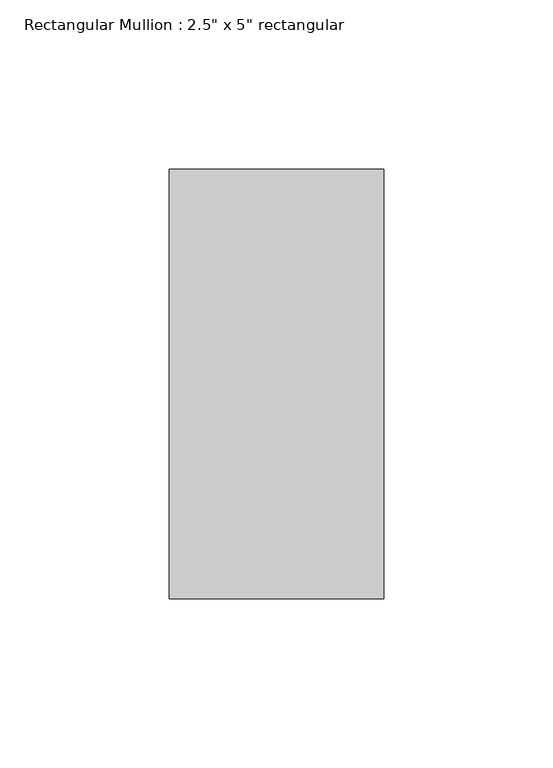
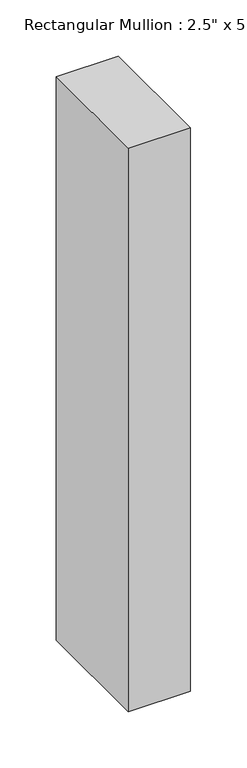
"""IFC4 building model written with IfcOpenShell, lengths in millimetres: member geometry."""

from ifc_helpers import new_model, si_unit, frame, origin, place, context, project, spatial, polyline, outline, extrude, source, transform, mapped, element, save


def member_47bfaf8a(model_context):
    return source(origin(), model_context, "Body", "SweptSolid", [
        extrude(outline(polyline([(0.0, 63.5), (0.0, -63.5), (-63.5, -63.5), (-63.5, 63.5), (0.0, 63.5)])), frame((0.0, 0.0, -609.6), z_axis=(0.0, 0.0, 1.0), x_axis=(1.0, 0.0, 0.0)), (0.0, 0.0, 1.0), 609.6),
    ])


if __name__ == "__main__":
    model = new_model("IFC4")
    model_context = context("Model", 3, world=origin())
    ifc_project = project(units=[si_unit("LENGTHUNIT", "METRE", prefix="MILLI")], contexts=[model_context])
    site = spatial("IfcSite", under=ifc_project)
    building = spatial("IfcBuilding", under=site)
    placement = place(None, origin())
    member_shape = member_47bfaf8a(model_context)
    element("IfcMember", 1, ObjectType="Rectangular Mullion : 2.5\" x 5\" rectangular", at=placement, inside=building, context=model_context, shape_type="MappedRepresentation", body=[
        mapped(member_shape, transform((0.0, 0.0, 0.0), x_axis=(1.0, 0.0, 0.0), y_axis=(0.0, 1.0, 0.0), z_axis=(0.0, 0.0, 1.0))),
    ])
    save(model, "model.ifc")

# Revit data of these elements
# Type "Rectangular Mullion : 2.5\" x 5\" rectangular"
#   built-in parameter 1007304 = 0.416667 (stored number, unit not read)
#   built-in parameter 1007301 = 0.104167 (stored number, unit not read)
#   built-in parameter 1007300 = 0.104167 (stored number, unit not read)
# Element 1 (IfcMember, "Rectangular Mullion : 2.5\" x 5\" rectangular")
#   Materials on its faces: "BLACK COLOUR"
# Materials
#   "BLACK COLOUR": class "Generic", colour RGB 120 120 120, transparency 0, Cost = 0
